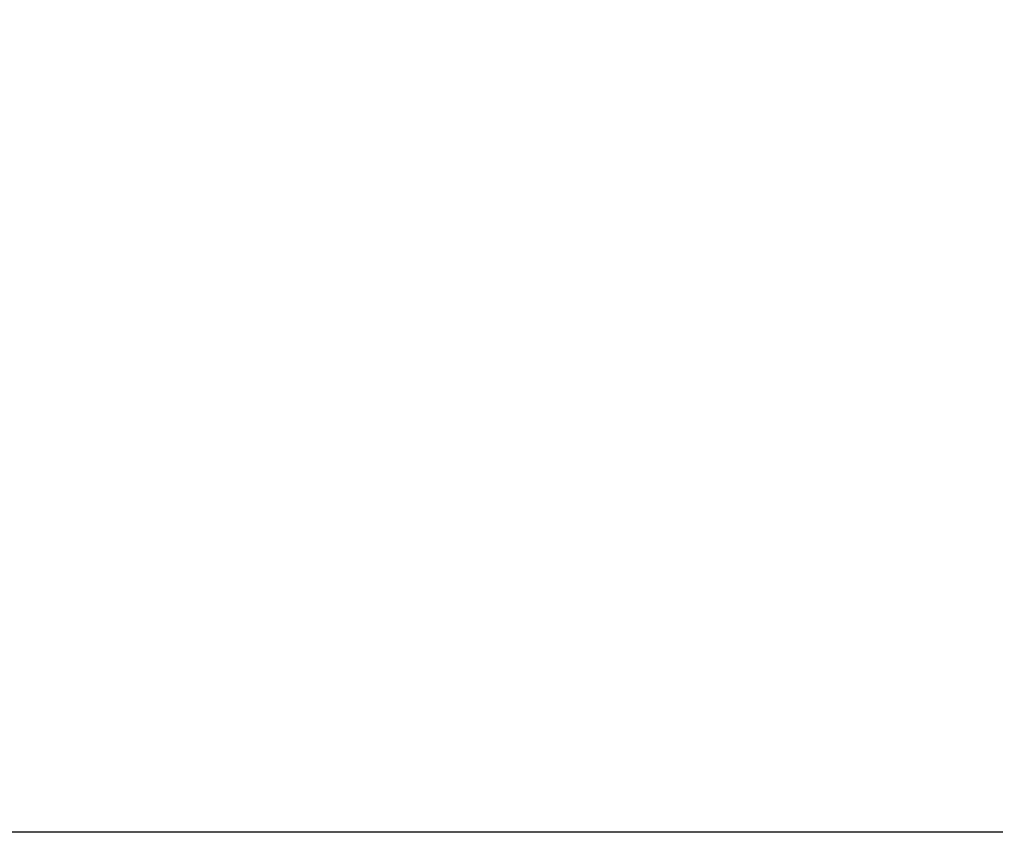
# Model space of a CAD drawing. Units: millimetres. Extents: x 0 to 2267, y 0 to 1823.
# Tile 6 of 256: x 1459 to 1506, y 1077 to 1116. Entities that reach past the tile are written whole.
import ezdxf

# ---------------------------------------------------------------- set-up
doc = ezdxf.new("R2010")
doc.units = ezdxf.units.MM
doc.header["$MEASUREMENT"] = 0
doc.layers.add('M-DIMS', color=2, linetype='Continuous', lineweight=25)
doc.styles.get("Standard").update_dxf_attribs({"font": 'arial.ttf'})
doc.dimstyles.get("Standard").update_dxf_attribs({"dimtxt": 7, "dimasz": 4, "dimexe": 0.18, "dimexo": 0.0625, "dimgap": 0.09, "dimtad": 0, "dimdec": 0, "dimzin": 0, "dimdsep": 46, "dimtxsty": 'Standard', "dimcen": 0.09, "dimadec": 0, "dimazin": 0, "dimtfac": 1, "dimtdec": 0, "dimtofl": 0, "dimtmove": 0, "dimatfit": 3, "dimfxl": 1, "dimtolj": 1, "dimtzin": 0, "dimarcsym": 0})

# ---------------------------------------------------------------- blocks, each defined once
blk = doc.blocks.new('*D9')
at = {"layer": 'Defpoints', "color": 0, "transparency": 16777216}
for p in [(1332.087, 1117.417), (1505.929, 1117.417), (1505.929, 1077.417)]:
    blk.add_point(p, dxfattribs=at)
at = {"layer": 'M-DIMS', "color": 0, "lineweight": -2, "transparency": 16777216}
for p, q in [((1505.866, 1117.417), (1331.907, 1117.417)), ((1332.087, 1113.417), (1332.087, 1102.65)), ((1332.087, 1081.417), (1332.087, 1092.184)), ((1505.866, 1077.417), (1331.907, 1077.417))]:
    blk.add_line(p, q, dxfattribs=at)
at = {"layer": 'M-DIMS', "color": 0, "transparency": 16777216}
for points in [[(1331.42, 1113.417), (1332.753, 1113.417), (1332.087, 1117.417)], [(1331.42, 1081.417), (1332.753, 1081.417), (1332.087, 1077.417)]]:
    blk.add_solid(points, dxfattribs=at)
at = {"layer": 'M-DIMS', "color": 0, "transparency": 16777216, "insert": (1332.087, 1097.417), "char_height": 7, "attachment_point": 5, "rotation": 90}
blk.add_mtext('\\A1;40', dxfattribs=at)

msp = doc.modelspace()

# ---------------------------------------------------------------- dimensions: what is measured, and where the dimension line sits
at = {"layer": 'M-DIMS'}
dim = msp.add_linear_dim(base=(1332.087, 1117.417), p1=(1505.929, 1077.417), p2=(1505.929, 1117.417), angle=90, dimstyle='Standard', override={"dimdec": 0, "dimlfac": 1, "dimrnd": 0, "dimzin": 0, "dimdsep": 46, "dimlunit": 2}, dxfattribs=at)
dim.commit()
dim.dimension.update_dxf_attribs({"geometry": '*D9', "text_midpoint": (1332.087, 1097.417)})

doc.saveas('drawing.dxf')
